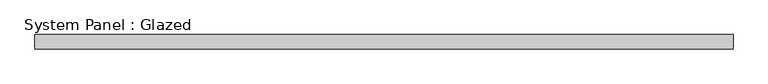
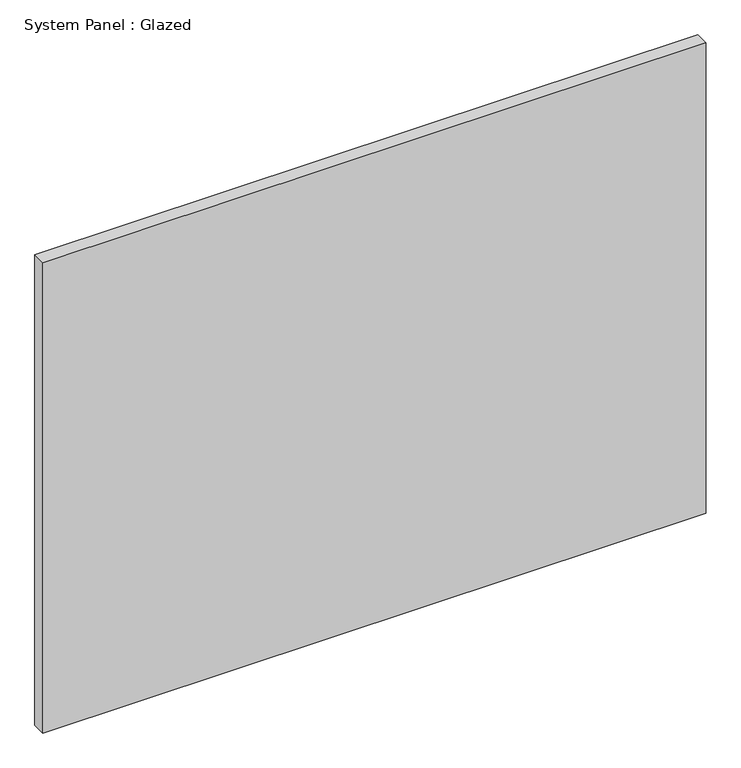
"""IFC4 building model written with IfcOpenShell, lengths in millimetres: plate geometry, System Panel : Glazed."""

from ifc_helpers import new_model, si_unit, origin, origin_with_axes, place, context, project, spatial, polyline, outline, extrude, source, transform, mapped, element, save


def system_panel_glazed_8b63b301(model_context):
    return source(origin(), model_context, "Body", "SweptSolid", [
        extrude(outline(polyline([(609.6, 19.05), (-609.6, 19.05), (-609.6, 44.45), (609.6, 44.45), (609.6, 19.05)])), origin_with_axes(), (0.0, 0.0, 1.0), 914.4),
    ])


if __name__ == "__main__":
    model = new_model("IFC4")
    model_context = context("Model", 3, world=origin())
    ifc_project = project(units=[si_unit("LENGTHUNIT", "METRE", prefix="MILLI")], contexts=[model_context])
    site = spatial("IfcSite", under=ifc_project)
    building = spatial("IfcBuilding", under=site)
    placement = place(None, origin())
    system_panel_glazed_shape = system_panel_glazed_8b63b301(model_context)
    element("IfcPlate", 1, ObjectType="System Panel : Glazed", at=placement, inside=building, context=model_context, shape_type="MappedRepresentation", body=[
        mapped(system_panel_glazed_shape, transform((0.0, 0.0, 0.0), x_axis=(1.0, 0.0, 0.0), y_axis=(0.0, 1.0, 0.0), z_axis=(0.0, 0.0, 1.0))),
    ])
    save(model, "model.ifc")

# Revit data of these elements
# Type "System Panel : Glazed"
#   Construction Type Id = "GSP4R"
#   Analytic Construction = "1/8 in Pilkington single glazing"
#   Visual Light Transmittance = 0.9
#   Solar Heat Gain Coefficient = 0.86
#   Heat Transfer Coefficient (U) = 1.18115 BTU/(h·ft²·°F)
# Element 1 (IfcPlate, "System Panel : Glazed")
#   Materials on its faces: "Glass"
# Materials
#   "Glass": class "Glass", colour RGB 0 128 192, transparency 0.75, Description = "Soda Lime Glass", Cost = 0
